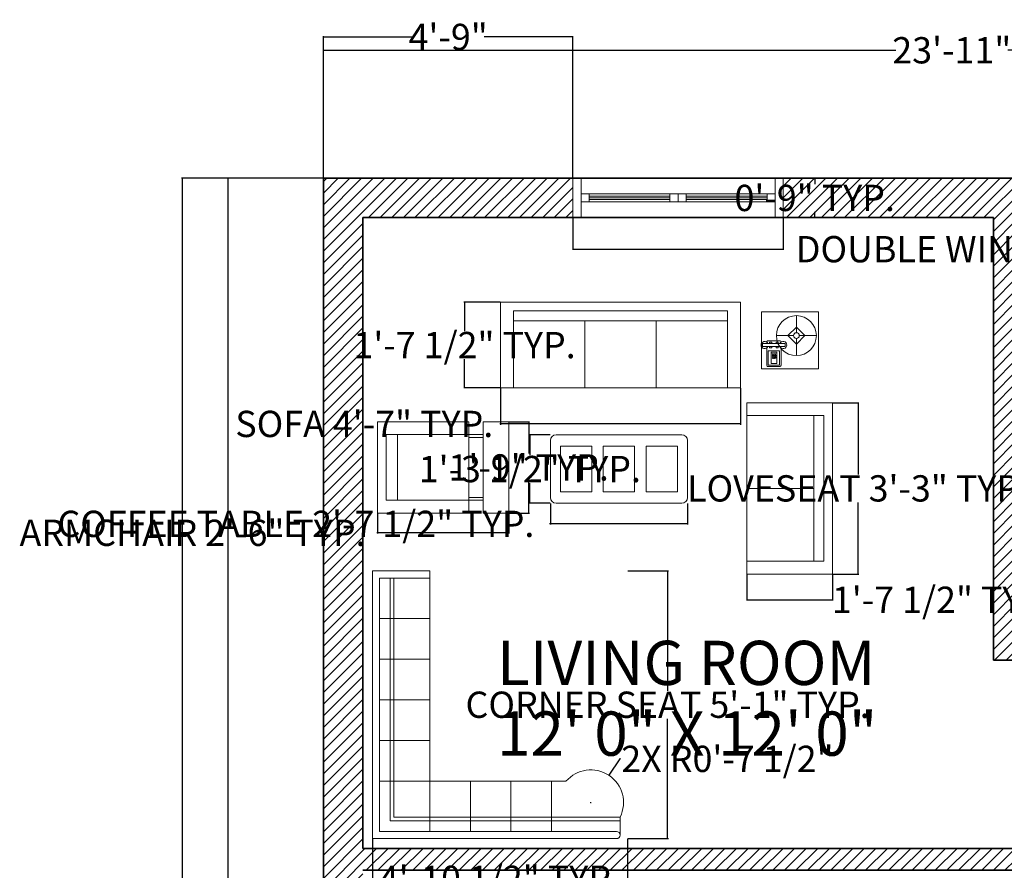
# Model space of a CAD drawing. Units: inches. Extents: x 585 to 1401, y -184 to 463.
# Tile 5 of 8: x 585 to 810, y 264 to 458. Entities that reach past the tile are written whole.
import ezdxf

# ---------------------------------------------------------------- set-up
doc = ezdxf.new("R2010")
doc.units = ezdxf.units.IN
doc.header["$MEASUREMENT"] = 0
for name, color, linetype, lineweight in [('A-ANNO-DIMS', 2, 'Continuous', 18), ('A-AREA-IDEN', 7, 'Continuous', 18), ('A-EQPM', 8, 'Continuous', 13), ('A-FURN', 8, 'Continuous', 18), ('A-Glaz', 140, 'Continuous', 18), ('A-Wall', 7, 'Continuous', 35), ('A-WALL-PATT', 252, 'Continuous', 13)]:
    doc.layers.add(name, color=color, linetype=linetype, lineweight=lineweight)
doc.styles.get("Standard").update_dxf_attribs({"font": 'arial.ttf'})
doc.dimstyles.get("Standard").update_dxf_attribs({"dimtxt": 6, "dimasz": 0.18, "dimexe": 0.18, "dimexo": 0.0625, "dimgap": 0.09, "dimtad": 0, "dimtih": 1, "dimtoh": 1, "dimdec": 0, "dimzin": 0, "dimdsep": 46, "dimlunit": 3, "dimtxsty": 'Standard', "dimblk": 'ARCHTICK', "dimcen": 0.09, "dimadec": 0, "dimazin": 0, "dimtfac": 1, "dimtdec": 0, "dimtofl": 0, "dimtmove": 0, "dimatfit": 3, "dimfxl": 1, "dimtolj": 1, "dimtzin": 0, "dimarcsym": 0})

# ---------------------------------------------------------------- blocks, each defined once
blk = doc.blocks.new('RECLIN32')
for p, q in [((16, 0), (16, -32)), ((-11.5, -3), (11.5, -3)), ((-11.5, -32), (-11.5, -3)), ((11.5, -3), (11.5, -32)), ((-11.5, -7), (11.5, -7)), ((-11.5, -32), (-11.5, -37)), ((-10.5, -32), (-10.5, -37)), ((10.5, -32), (10.5, -37)), ((11.5, -32), (11.5, -37))]:
    blk.add_line(p, q)
blk.add_lwpolyline([(16, -32), (-16, -32), (-16, 0), (16, 0)])
blk.add_lwpolyline([(-16, -46), (-16, -37), (16, -37), (16, -46)], close=True)
blk = doc.blocks.new('LOVESET5')
for p, q in [((35.75, 0), (35.75, -30.00001)), ((-19.75, -3), (31.25, -3)), ((-19.75, -30.00001), (-19.75, -3)), ((31.25, -3), (31.25, -30.00001)), ((-19.75, -6.5), (31.25, -6.5)), ((5.75, -6.5), (5.75, -30.00001))]:
    blk.add_line(p, q)
for points in [[(35.75, -30.00001), (-24.25, -30.00001), (-24.25, 0), (24.25, 0)], [(24.25, 0), (35.75, 0)]]:
    blk.add_lwpolyline(points)
blk = doc.blocks.new('TBLEN20S')
blk.add_lwpolyline([(-10, -10), (-10, 10), (10, 10), (10, -10)], close=True)
blk = doc.blocks.new('LAMP')
for p, q in [((0, 7), (0, 1)), ((-1, 0), (-7, 0)), ((0, 3), (-3, 0)), ((-3, 0), (0, -3)), ((3, 0), (0, 3)), ((0, -3), (3, 0)), ((1, 0), (7, 0)), ((0, -1), (0, -7))]:
    blk.add_line(p, q)
for radius in [7, 1]:
    blk.add_circle((0, 0), radius)
blk = doc.blocks.new('SOFA7')
for p, q in [((-37.5, -3), (37.5, -3)), ((-37.5, -30), (-37.5, -3)), ((37.5, -3), (37.5, -30)), ((-37.5, -6.5), (37.5, -6.5)), ((-12.5, -6.5), (-12.5, -30)), ((12.5, -6.5), (12.5, -30))]:
    blk.add_line(p, q)
blk.add_lwpolyline([(-42, -30), (-42, 0), (42, 0), (42, -30)], close=True)
blk = doc.blocks.new('TBLWGLAS')
for p, q in [((-22, 0), (22, 0)), ((-24, -22), (-24, -2)), ((24, -2), (24, -22)), ((-20.5, -20), (-20.5, -4)), ((-20.5, -4), (-9.5, -4)), ((-9.5, -4), (-9.5, -20)), ((-5.5, -20), (-5.5, -4)), ((-5.5, -4), (5.5, -4)), ((5.5, -4), (5.5, -20)), ((9.5, -20), (9.5, -4)), ((9.5, -4), (20.5, -4)), ((20.5, -4), (20.5, -20)), ((-9.5, -20), (-20.5, -20)), ((5.5, -20), (-5.5, -20)), ((20.5, -20), (9.5, -20)), ((22, -24), (-22, -24))]:
    blk.add_line(p, q)
for centre, start, end in [((-22, -2), 90, 180), ((22, -2), 0, 90), ((-22, -22), 180, 270), ((22, -22), 270, 0)]:
    blk.add_arc(centre, 2, start, end)
blk = doc.blocks.new('PHONE')
for p, q in [((-3.99, 3.5), (-3.99, 2.5)), ((4.01, 3.5), (-3.99, 3.5)), ((-2.02, 4.5), (2.02, 4.5)), ((-1.49, 4), (-0.74, 4)), ((-1.49, 3.5), (-1.49, 4)), ((-0.74, 4), (-0.74, 3.5)), ((0.76, 4), (0.76, 3.5)), ((1.51, 4), (0.76, 4)), ((1.51, 3.5), (1.51, 4)), ((4.01, 2.5), (4.01, 3.5)), ((-3.99, 2.5), (4.01, 2.5)), ((-2.49, -4.03), (-2.49, 1.92)), ((-1.99, 1), (-1.99, -4)), ((2.01, 1), (-1.99, 1)), ((-1.49, 2), (-1.49, 2.5)), ((-0.74, 2), (-1.49, 2)), ((1.01, 0.5), (-0.99, 0.5)), ((-0.99, 0.5), (-0.99, -3.5)), ((-0.74, 2.5), (-0.74, 2)), ((0.76, 2.5), (0.76, 2)), ((0.76, 2), (1.51, 2)), ((1.01, -3.5), (1.01, 0.5)), ((1.51, 2), (1.51, 2.5)), ((2.01, -4), (2.01, 1)), ((2.51, 1.95), (2.51, -4.06)), ((2.04, -4.5), (-2.01, -4.5)), ((-1.99, -4), (2.01, -4)), ((-0.99, -3.5), (1.01, -3.5))]:
    blk.add_line(p, q)
for centre, radius, start, end in [((-3.24, 3), 1.27, 24.0275, 336.6167), ((-2.05, 4.06), 0.442, 81.8699, 188.1301), ((2.07, 4.06), 0.442, 351.8699, 98.1301), ((3.26, 3), 1.25, 205.0096, 154.8206), ((-2.05, -4.06), 0.442, 171.8699, 278.1301), ((2.07, -4.06), 0.442, 261.8699, 8.1301)]:
    blk.add_arc(centre, radius, start, end)
blk = doc.blocks.new('QU')
at = {"color": 0}
for p, q in [((-0.8, -2.5), (-0.8, 1.233)), ((-0.8, 1.233), (0, 1.233)), ((-0.7, -2.4), (-0.7, 1.133)), ((-0.7, 1.133), (0, 1.133)), ((-0.55, -2.25), (-0.55, 1.133)), ((-0.5, -2.2), (-0.5, 1.133)), ((0, 1.233), (0, -2.4)), ((-0.7, 0.567), (0, 0.567)), ((-0.7, 0), (0, 0)), ((-0.7, -0.567), (0, -0.567)), ((-0.7, -1.133), (0, -1.133)), ((-0.7, -1.7), (1.133, -1.7)), ((-0.133, -1.7), (1.7, -1.7)), ((0.567, -1.7), (0.567, -2.4)), ((1.133, -1.7), (1.133, -2.4)), ((1.133, -1.7), (1.133, -2.4)), ((1.7, -1.7), (1.9, -1.7)), ((1.7, -1.7), (1.7, -2.4)), ((2.655, -2.25), (-0.55, -2.25)), ((2.655, -2.2), (-0.5, -2.2)), ((2.655, -2.45), (2.655, -2.2)), ((2.605, -2.4), (-0.7, -2.4)), ((2.605, -2.5), (-0.8, -2.5))]:
    blk.add_line(p, q, dxfattribs=at)
for centre, radius, start, end in [((2.247, -1.997), 0.456, 333.5922, 139.3979), ((2.605, -2.45), 0.05, 270, 90)]:
    blk.add_arc(centre, radius, start, end, dxfattribs=at)
blk = doc.blocks.new('_ArchTick')
at = {"color": 0, "linetype": 'ByBlock', "const_width": 0.15}
blk.add_lwpolyline([(-0.5, -0.5), (0.5, 0.5)], dxfattribs=at)
blk = doc.blocks.new('*D27')
at = {"layer": 'A-ANNO-DIMS', "color": 0, "lineweight": -2, "transparency": 16777216}
for p, q in [((654.47, 422.15), (632.54, 422.15)), ((632.72, 422.15), (632.72, 159.24)), ((632.72, -109.85), (632.72, 153.06)), ((654.47, -109.85), (632.54, -109.85))]:
    blk.add_line(p, q, dxfattribs=at)
at = {"layer": 'Defpoints', "color": 0, "transparency": 16777216}
for p in [(654.53, 422.15), (632.72, -109.85), (654.53, -109.85)]:
    blk.add_point(p, dxfattribs=at)
at = {"layer": 'A-ANNO-DIMS', "color": 0, "lineweight": -2, "transparency": 16777216, "xscale": 0.18, "yscale": 0.18, "zscale": 0.18}
for p, rotation in [((632.72, 422.15), 90), ((632.72, -109.85), 270)]:
    blk.add_blockref('_ArchTick', p, dxfattribs=dict(at, rotation=rotation))
at = {"layer": 'A-ANNO-DIMS', "color": 0, "transparency": 16777216, "insert": (632.72, 156.15), "char_height": 6, "attachment_point": 5}
blk.add_mtext('\\A1;44\'-4"', dxfattribs=at)
blk = doc.blocks.new('*D28')
at = {"layer": 'A-ANNO-DIMS', "color": 0, "lineweight": -2, "transparency": 16777216}
for p, q in [((654.53, 422.22), (654.53, 451.54)), ((654.53, 451.36), (785.25, 451.36)), ((941.53, 451.36), (810.81, 451.36)), ((941.53, 422.22), (941.53, 451.54))]:
    blk.add_line(p, q, dxfattribs=at)
at = {"layer": 'Defpoints', "color": 0, "transparency": 16777216}
for p in [(941.53, 451.36), (654.53, 422.15), (941.53, 422.15)]:
    blk.add_point(p, dxfattribs=at)
at = {"layer": 'A-ANNO-DIMS', "color": 0, "lineweight": -2, "transparency": 16777216, "xscale": 0.18, "yscale": 0.18, "zscale": 0.18, "rotation": 180}
blk.add_blockref('_ArchTick', (654.53, 451.36), dxfattribs=at)
at = {"layer": 'A-ANNO-DIMS', "color": 0, "lineweight": -2, "transparency": 16777216, "xscale": 0.18, "yscale": 0.18, "zscale": 0.18}
blk.add_blockref('_ArchTick', (941.53, 451.36), dxfattribs=at)
at = {"layer": 'A-ANNO-DIMS', "color": 0, "transparency": 16777216, "insert": (798.03, 451.36), "char_height": 6, "attachment_point": 5}
blk.add_mtext('\\A1;23\'-11"', dxfattribs=at)
blk = doc.blocks.new('WIN-48-DOUBLE-PANEL')
for p, q in [((48, 9), (0, 9)), ((0, 9), (0, 0)), ((1.85, 9), (0, 9)), ((0, 9), (0, 0)), ((1.85, 0), (1.85, 9)), ((1.85, 0), (1.85, 9)), ((46.15, 9), (48, 9)), ((46.15, 0), (46.15, 9)), ((46.15, 0), (46.15, 9)), ((46.15, 0), (46.15, 9)), ((48, 9), (48, 0)), ((48, 0), (48, 9)), ((1.85, 5.44), (46.15, 5.44)), ((3.69, 3.6), (3.69, 5.44)), ((3.69, 4.89), (22.15, 4.89)), ((3.69, 4.52), (22.15, 4.52)), ((22.15, 5.44), (22.15, 3.6)), ((24, 5.44), (24, 3.6)), ((25.85, 5.44), (25.85, 3.6)), ((44.31, 4.89), (25.85, 4.89)), ((44.31, 4.52), (25.85, 4.52)), ((44.31, 3.6), (44.31, 5.44)), ((1.85, 3.6), (46.15, 3.6)), ((3.69, 4.15), (22.15, 4.15)), ((44.31, 4.15), (25.85, 4.15)), ((0, 0), (1.85, 0)), ((48, 0), (0, 0)), ((48, 0), (46.15, 0))]:
    blk.add_line(p, q)
blk = doc.blocks.new('TELEPHONE-KEYPAD')
for centre in [(0.08, 1.02), (0.11, 0.71), (0.14, 0.39), (0.15, 0.09), (0.39, 1.03), (0.42, 0.71), (0.41, 0.38), (0.44, 0.08), (0.73, 1.02), (0.74, 0.7), (0.75, 0.4), (0.76, 0.13)]:
    blk.add_circle(centre, 0.0754)
blk = doc.blocks.new('*D38')
at = {"layer": 'A-ANNO-DIMS', "color": 0, "lineweight": -2, "transparency": 16777216}
for p, q in [((711.53, 413.09), (711.53, 405.77)), ((759.53, 413.09), (759.53, 405.77)), ((711.53, 405.95), (759.53, 405.95)), ((759.53, 405.95), (759.71, 405.95))]:
    blk.add_line(p, q, dxfattribs=at)
at = {"layer": 'Defpoints', "color": 0, "transparency": 16777216}
for p in [(711.53, 413.15), (759.53, 413.15), (759.53, 405.95)]:
    blk.add_point(p, dxfattribs=at)
at = {"layer": 'A-ANNO-DIMS', "color": 0, "lineweight": -2, "transparency": 16777216, "xscale": 0.18, "yscale": 0.18, "zscale": 0.18, "rotation": 180}
blk.add_blockref('_ArchTick', (711.53, 405.95), dxfattribs=at)
at = {"layer": 'A-ANNO-DIMS', "color": 0, "lineweight": -2, "transparency": 16777216, "xscale": 0.18, "yscale": 0.18, "zscale": 0.18}
blk.add_blockref('_ArchTick', (759.53, 405.95), dxfattribs=at)
at = {"layer": 'A-ANNO-DIMS', "color": 0, "transparency": 16777216, "insert": (815.89, 405.95), "char_height": 6, "attachment_point": 5}
blk.add_mtext('\\A1;DOUBLE WINDOW 4\'-0" TYP.', dxfattribs=at)
blk = doc.blocks.new('*D39')
at = {"layer": 'A-ANNO-DIMS', "color": 0, "lineweight": -2, "transparency": 16777216}
for p, q in [((759.59, 422.15), (766.91, 422.15)), ((766.73, 422.15), (766.73, 420.81)), ((766.73, 413.15), (766.73, 414.5)), ((759.59, 413.15), (766.91, 413.15))]:
    blk.add_line(p, q, dxfattribs=at)
at = {"layer": 'Defpoints', "color": 0, "transparency": 16777216}
for p in [(759.53, 422.15), (766.73, 422.15), (759.53, 413.15)]:
    blk.add_point(p, dxfattribs=at)
at = {"layer": 'A-ANNO-DIMS', "color": 0, "lineweight": -2, "transparency": 16777216, "xscale": 0.18, "yscale": 0.18, "zscale": 0.18}
for p, rotation in [((766.73, 422.15), 90), ((766.73, 413.15), 270)]:
    blk.add_blockref('_ArchTick', p, dxfattribs=dict(at, rotation=rotation))
at = {"layer": 'A-ANNO-DIMS', "color": 0, "transparency": 16777216, "insert": (766.73, 417.65), "char_height": 6, "attachment_point": 5}
blk.add_mtext('\\A1;0\'-9" TYP.', dxfattribs=at)
blk = doc.blocks.new('*D48')
at = {"layer": 'A-ANNO-DIMS', "color": 0, "lineweight": -2, "transparency": 16777216}
for p, q in [((666.91, 345.64), (666.91, 341.02)), ((696.91, 345.64), (696.91, 341.02)), ((666.91, 341.2), (666.73, 341.2)), ((696.91, 341.2), (666.91, 341.2))]:
    blk.add_line(p, q, dxfattribs=at)
at = {"layer": 'Defpoints', "color": 0, "transparency": 16777216}
for p in [(666.91, 345.7), (696.91, 345.7), (666.91, 341.2)]:
    blk.add_point(p, dxfattribs=at)
at = {"layer": 'A-ANNO-DIMS', "color": 0, "lineweight": -2, "transparency": 16777216, "xscale": 0.18, "yscale": 0.18, "zscale": 0.18, "rotation": 180.0000000000005}
blk.add_blockref('_ArchTick', (666.91, 341.2), dxfattribs=at)
at = {"layer": 'A-ANNO-DIMS', "color": 0, "lineweight": -2, "transparency": 16777216, "xscale": 0.18, "yscale": 0.18, "zscale": 0.18}
blk.add_blockref('_ArchTick', (696.91, 341.2), dxfattribs=at)
at = {"layer": 'A-ANNO-DIMS', "color": 0, "transparency": 16777216, "insert": (624.66, 341.2), "char_height": 6, "attachment_point": 5}
blk.add_mtext('\\A1;ARMCHAIR 2\'-6" TYP.', dxfattribs=at)
blk = doc.blocks.new('*D49')
at = {"layer": 'A-ANNO-DIMS', "color": 0, "lineweight": -2, "transparency": 16777216}
for p, q in [((696.97, 366.57), (701.59, 366.57)), ((701.41, 366.57), (701.41, 359.29)), ((701.41, 345.7), (701.41, 352.98)), ((696.97, 345.7), (701.59, 345.7))]:
    blk.add_line(p, q, dxfattribs=at)
at = {"layer": 'Defpoints', "color": 0, "transparency": 16777216}
for p in [(696.91, 366.57), (696.91, 345.7), (701.41, 345.7)]:
    blk.add_point(p, dxfattribs=at)
at = {"layer": 'A-ANNO-DIMS', "color": 0, "lineweight": -2, "transparency": 16777216, "xscale": 0.18, "yscale": 0.18, "zscale": 0.18}
for p, rotation in [((701.41, 366.57), 90), ((701.41, 345.7), 270)]:
    blk.add_blockref('_ArchTick', p, dxfattribs=dict(at, rotation=rotation))
at = {"layer": 'A-ANNO-DIMS', "color": 0, "transparency": 16777216, "insert": (701.41, 356.13), "char_height": 6, "attachment_point": 5}
blk.add_mtext('\\A1;1\'-9" TYP.', dxfattribs=at)
blk = doc.blocks.new('*D50')
at = {"layer": 'A-ANNO-DIMS', "color": 0, "lineweight": -2, "transparency": 16777216}
for p, q in [((770.82, 370.91), (776.81, 370.91)), ((776.63, 370.91), (776.63, 354.54)), ((776.63, 331.78), (776.63, 348.14)), ((770.82, 331.78), (776.81, 331.78))]:
    blk.add_line(p, q, dxfattribs=at)
at = {"layer": 'Defpoints', "color": 0, "transparency": 16777216}
for p in [(770.76, 370.91), (776.63, 370.91), (770.76, 331.78)]:
    blk.add_point(p, dxfattribs=at)
at = {"layer": 'A-ANNO-DIMS', "color": 0, "lineweight": -2, "transparency": 16777216, "xscale": 0.18, "yscale": 0.18, "zscale": 0.18}
for p, rotation in [((776.63, 370.91), 90), ((776.63, 331.78), 270)]:
    blk.add_blockref('_ArchTick', p, dxfattribs=dict(at, rotation=rotation))
at = {"layer": 'A-ANNO-DIMS', "color": 0, "transparency": 16777216, "insert": (776.63, 351.34), "char_height": 6, "attachment_point": 5}
blk.add_mtext('\\A1;LOVESEAT 3\'-3" TYP.', dxfattribs=at)
blk = doc.blocks.new('*D51')
at = {"layer": 'A-ANNO-DIMS', "color": 0, "lineweight": -2, "transparency": 16777216}
for p, q in [((751.2, 331.71), (751.2, 325.73)), ((770.76, 331.71), (770.76, 325.73)), ((751.2, 325.91), (770.76, 325.91)), ((770.76, 325.91), (770.94, 325.91))]:
    blk.add_line(p, q, dxfattribs=at)
at = {"layer": 'Defpoints', "color": 0, "transparency": 16777216}
for p in [(751.2, 331.78), (770.76, 331.78), (770.76, 325.91)]:
    blk.add_point(p, dxfattribs=at)
at = {"layer": 'A-ANNO-DIMS', "color": 0, "lineweight": -2, "transparency": 16777216, "xscale": 0.18, "yscale": 0.18, "zscale": 0.18, "rotation": 180}
blk.add_blockref('_ArchTick', (751.2, 325.91), dxfattribs=at)
at = {"layer": 'A-ANNO-DIMS', "color": 0, "lineweight": -2, "transparency": 16777216, "xscale": 0.18, "yscale": 0.18, "zscale": 0.18}
blk.add_blockref('_ArchTick', (770.76, 325.91), dxfattribs=at)
at = {"layer": 'A-ANNO-DIMS', "color": 0, "transparency": 16777216, "insert": (796.03, 325.91), "char_height": 6, "attachment_point": 5}
blk.add_mtext('\\A1;1\'-7 1/2" TYP.', dxfattribs=at)
blk = doc.blocks.new('*D56')
at = {"layer": 'A-ANNO-DIMS', "color": 0, "lineweight": -2, "transparency": 16777216}
for p, q in [((694.99, 374.21), (694.99, 365.88)), ((749.77, 374.21), (749.77, 365.88)), ((694.99, 366.06), (694.81, 366.06)), ((749.77, 366.06), (694.99, 366.06))]:
    blk.add_line(p, q, dxfattribs=at)
at = {"layer": 'Defpoints', "color": 0, "transparency": 16777216}
for p in [(694.99, 374.27), (749.77, 374.27), (694.99, 366.06)]:
    blk.add_point(p, dxfattribs=at)
at = {"layer": 'A-ANNO-DIMS', "color": 0, "lineweight": -2, "transparency": 16777216, "xscale": 0.18, "yscale": 0.18, "zscale": 0.18, "rotation": 180}
blk.add_blockref('_ArchTick', (694.99, 366.06), dxfattribs=at)
at = {"layer": 'A-ANNO-DIMS', "color": 0, "lineweight": -2, "transparency": 16777216, "xscale": 0.18, "yscale": 0.18, "zscale": 0.18}
blk.add_blockref('_ArchTick', (749.77, 366.06), dxfattribs=at)
at = {"layer": 'A-ANNO-DIMS', "color": 0, "transparency": 16777216, "insert": (663.87, 366.06), "char_height": 6, "attachment_point": 5}
blk.add_mtext('\\A1;SOFA 4\'-7" TYP.', dxfattribs=at)
blk = doc.blocks.new('*D57')
at = {"layer": 'A-ANNO-DIMS', "color": 0, "lineweight": -2, "transparency": 16777216}
for p, q in [((694.93, 393.84), (686.59, 393.84)), ((686.77, 393.84), (686.77, 387.25)), ((686.77, 374.27), (686.77, 380.86)), ((694.93, 374.27), (686.59, 374.27))]:
    blk.add_line(p, q, dxfattribs=at)
at = {"layer": 'Defpoints', "color": 0, "transparency": 16777216}
for p in [(686.77, 393.84), (694.99, 393.84), (694.99, 374.27)]:
    blk.add_point(p, dxfattribs=at)
at = {"layer": 'A-ANNO-DIMS', "color": 0, "lineweight": -2, "transparency": 16777216, "xscale": 0.18, "yscale": 0.18, "zscale": 0.18}
for p, rotation in [((686.77, 393.84), 90), ((686.77, 374.27), 270)]:
    blk.add_blockref('_ArchTick', p, dxfattribs=dict(at, rotation=rotation))
at = {"layer": 'A-ANNO-DIMS', "color": 0, "transparency": 16777216, "insert": (686.77, 384.06), "char_height": 6, "attachment_point": 5}
blk.add_mtext('\\A1;1\'-7 1/2" TYP.', dxfattribs=at)
blk = doc.blocks.new('*D58')
at = {"layer": 'A-ANNO-DIMS', "color": 0, "lineweight": -2, "transparency": 16777216}
for p, q in [((706.37, 347.87), (706.37, 343.06)), ((737.67, 347.87), (737.67, 343.06)), ((706.37, 343.24), (706.19, 343.24)), ((737.67, 343.24), (706.37, 343.24))]:
    blk.add_line(p, q, dxfattribs=at)
at = {"layer": 'Defpoints', "color": 0, "transparency": 16777216}
for p in [(706.37, 347.93), (737.67, 347.93), (706.37, 343.24)]:
    blk.add_point(p, dxfattribs=at)
at = {"layer": 'A-ANNO-DIMS', "color": 0, "lineweight": -2, "transparency": 16777216, "xscale": 0.18, "yscale": 0.18, "zscale": 0.18, "rotation": 180}
blk.add_blockref('_ArchTick', (706.37, 343.24), dxfattribs=at)
at = {"layer": 'A-ANNO-DIMS', "color": 0, "lineweight": -2, "transparency": 16777216, "xscale": 0.18, "yscale": 0.18, "zscale": 0.18}
blk.add_blockref('_ArchTick', (737.67, 343.24), dxfattribs=at)
at = {"layer": 'A-ANNO-DIMS', "color": 0, "transparency": 16777216, "insert": (648.25, 343.24), "char_height": 6, "attachment_point": 5}
blk.add_mtext('\\A1;COFFEE TABLE 2\'-7 1/2" TYP.', dxfattribs=at)
blk = doc.blocks.new('*D59')
at = {"layer": 'A-ANNO-DIMS', "color": 0, "lineweight": -2, "transparency": 16777216}
for p, q in [((706.3, 363.59), (701.49, 363.59)), ((701.67, 363.59), (701.67, 358.95)), ((701.67, 347.93), (701.67, 352.57)), ((706.3, 347.93), (701.49, 347.93))]:
    blk.add_line(p, q, dxfattribs=at)
at = {"layer": 'Defpoints', "color": 0, "transparency": 16777216}
for p in [(701.67, 363.59), (706.37, 363.59), (706.37, 347.93)]:
    blk.add_point(p, dxfattribs=at)
at = {"layer": 'A-ANNO-DIMS', "color": 0, "lineweight": -2, "transparency": 16777216, "xscale": 0.18, "yscale": 0.18, "zscale": 0.18}
for p, rotation in [((701.67, 363.59), 90), ((701.67, 347.93), 270)]:
    blk.add_blockref('_ArchTick', p, dxfattribs=dict(at, rotation=rotation))
at = {"layer": 'A-ANNO-DIMS', "color": 0, "transparency": 16777216, "insert": (701.67, 355.76), "char_height": 6, "attachment_point": 5}
blk.add_mtext('\\A1;1\'-3 1/2" TYP.', dxfattribs=at)
blk = doc.blocks.new('*D64')
at = {"layer": 'A-ANNO-DIMS', "color": 0, "lineweight": -2, "transparency": 16777216}
for p, q in [((724.03, 332.51), (733.32, 332.51)), ((733.14, 332.51), (733.14, 305.14)), ((733.14, 271.38), (733.14, 298.75)), ((724.03, 271.38), (733.32, 271.38))]:
    blk.add_line(p, q, dxfattribs=at)
at = {"layer": 'Defpoints', "color": 0, "transparency": 16777216}
for p in [(723.97, 332.51), (733.14, 332.51), (723.97, 271.38)]:
    blk.add_point(p, dxfattribs=at)
at = {"layer": 'A-ANNO-DIMS', "color": 0, "lineweight": -2, "transparency": 16777216, "xscale": 0.18, "yscale": 0.18, "zscale": 0.18}
for p, rotation in [((733.14, 332.51), 90), ((733.14, 271.38), 270)]:
    blk.add_blockref('_ArchTick', p, dxfattribs=dict(at, rotation=rotation))
at = {"layer": 'A-ANNO-DIMS', "color": 0, "transparency": 16777216, "insert": (733.14, 301.95), "char_height": 6, "attachment_point": 5}
blk.add_mtext('\\A1;CORNER SEAT 5\'-1" TYP.', dxfattribs=at)
blk = doc.blocks.new('*D65')
at = {"layer": 'A-ANNO-DIMS', "color": 0, "lineweight": -2, "transparency": 16777216}
for p, q in [((665.71, 271.32), (665.71, 262.03)), ((723.97, 271.32), (723.97, 262.03)), ((665.71, 262.21), (667.02, 262.21)), ((723.97, 262.21), (722.66, 262.21))]:
    blk.add_line(p, q, dxfattribs=at)
at = {"layer": 'Defpoints', "color": 0, "transparency": 16777216}
for p in [(665.71, 271.38), (723.97, 271.38), (723.97, 262.21)]:
    blk.add_point(p, dxfattribs=at)
at = {"layer": 'A-ANNO-DIMS', "color": 0, "lineweight": -2, "transparency": 16777216, "xscale": 0.18, "yscale": 0.18, "zscale": 0.18, "rotation": 180}
blk.add_blockref('_ArchTick', (665.71, 262.21), dxfattribs=at)
at = {"layer": 'A-ANNO-DIMS', "color": 0, "lineweight": -2, "transparency": 16777216, "xscale": 0.18, "yscale": 0.18, "zscale": 0.18}
blk.add_blockref('_ArchTick', (723.97, 262.21), dxfattribs=at)
at = {"layer": 'A-ANNO-DIMS', "color": 0, "transparency": 16777216, "insert": (694.84, 262.21), "char_height": 6, "attachment_point": 5}
blk.add_mtext('\\A1;4\'-10 1/2" TYP.', dxfattribs=at)
blk = doc.blocks.new('*D76')
at = {"layer": 'A-ANNO-DIMS', "color": 0, "lineweight": -2, "transparency": 16777216}
for p, q in [((654.47, 422.15), (622.1, 422.15)), ((622.28, 422.15), (622.28, 142.65)), ((622.28, -143.23), (622.28, 136.27)), ((807.47, -143.23), (622.1, -143.23))]:
    blk.add_line(p, q, dxfattribs=at)
at = {"layer": 'Defpoints', "color": 0, "transparency": 16777216}
for p in [(622.28, 422.15), (654.53, 422.15), (807.53, -143.23)]:
    blk.add_point(p, dxfattribs=at)
at = {"layer": 'A-ANNO-DIMS', "color": 0, "lineweight": -2, "transparency": 16777216, "xscale": 0.18, "yscale": 0.18, "zscale": 0.18}
for p, rotation in [((622.28, 422.15), 90), ((622.28, -143.23), 270)]:
    blk.add_blockref('_ArchTick', p, dxfattribs=dict(at, rotation=rotation))
at = {"layer": 'A-ANNO-DIMS', "color": 0, "transparency": 16777216, "insert": (622.28, 139.46), "char_height": 6, "attachment_point": 5}
blk.add_mtext('\\A1;47\'-1 1/2"', dxfattribs=at)
blk = doc.blocks.new('*D82')
at = {"layer": 'A-ANNO-DIMS', "color": 0, "lineweight": -2, "transparency": 16777216}
for p, q in [((654.53, 422.22), (654.53, 454.58)), ((654.53, 454.4), (674.84, 454.4)), ((711.53, 454.4), (691.21, 454.4)), ((711.53, 422.22), (711.53, 454.58))]:
    blk.add_line(p, q, dxfattribs=at)
at = {"layer": 'Defpoints', "color": 0, "transparency": 16777216}
for p in [(711.53, 454.4), (654.53, 422.15), (711.53, 422.15)]:
    blk.add_point(p, dxfattribs=at)
at = {"layer": 'A-ANNO-DIMS', "color": 0, "lineweight": -2, "transparency": 16777216, "xscale": 0.18, "yscale": 0.18, "zscale": 0.18, "rotation": 180}
blk.add_blockref('_ArchTick', (654.53, 454.4), dxfattribs=at)
at = {"layer": 'A-ANNO-DIMS', "color": 0, "lineweight": -2, "transparency": 16777216, "xscale": 0.18, "yscale": 0.18, "zscale": 0.18}
blk.add_blockref('_ArchTick', (711.53, 454.4), dxfattribs=at)
at = {"layer": 'A-ANNO-DIMS', "color": 0, "transparency": 16777216, "insert": (683.03, 454.4), "char_height": 6, "attachment_point": 5}
blk.add_mtext('\\A1;4\'-9"', dxfattribs=at)
blk = doc.blocks.new('*D98')
at = {"layer": 'A-ANNO-DIMS', "color": 0, "lineweight": -2, "transparency": 16777216}
for p, q in [((722.2, 289.59), (719.72, 285.85)), ((722.38, 289.59), (722.2, 289.59)), ((715.51, 279.62), (715.69, 279.62)), ((715.6, 279.53), (715.6, 279.71))]:
    blk.add_line(p, q, dxfattribs=at)
at = {"layer": 'Defpoints', "color": 0, "transparency": 16777216}
for p in [(719.72, 285.85), (715.6, 279.62)]:
    blk.add_point(p, dxfattribs=at)
at = {"layer": 'A-ANNO-DIMS', "color": 0, "lineweight": -2, "transparency": 16777216, "xscale": 0.18, "yscale": 0.18, "zscale": 0.18, "rotation": 236.4909758134295}
blk.add_blockref('_ArchTick', (719.72, 285.85), dxfattribs=at)
at = {"layer": 'A-ANNO-DIMS', "color": 0, "transparency": 16777216, "insert": (746.8, 289.59), "char_height": 6, "attachment_point": 5}
blk.add_mtext('\\A1;2X R0\'-7 1/2"', dxfattribs=at)

msp = doc.modelspace()

# ---------------------------------------------------------------- hatches: boundary and pattern name
at = {"layer": 'A-WALL-PATT'}
h = msp.add_hatch(dxfattribs=at)
h.set_pattern_fill('ANSI31', color=256, scale=15)
h.set_pattern_definition([(45, (599.059, -1e-14), (-1.325825, 1.325825), [])])
h.paths.add_polyline_path([(711.53, 422.15), (654.53, 422.15), (654.53, -109.85), (680.03, -109.85), (680.03, -100.85), (663.53, -100.85), (663.53, 48.87), (759.53, 48.87), (759.53, 57.87), (663.53, 57.87), (663.53, 144.15), (663.53, 264.15), (812.53, 264.15), (812.53, 269.15), (663.53, 269.15), (663.53, 413.15), (711.53, 413.15)])
h.paths.add_polyline_path([(753.53, -100.85), (728.03, -100.85), (728.03, -109.85), (753.53, -109.85)], flags=17)
h.paths.add_polyline_path([(812.53, -71.54), (807.53, -71.54), (807.53, -100.85), (795.53, -100.85), (795.53, -109.85), (807.53, -109.85), (807.53, -143.23), (848.53, -143.23), (848.53, -134.23), (812.53, -134.23)])
h.paths.add_polyline_path([(941.53, 8.77), (932.53, 8.77), (932.53, -9.23), (812.53, -9.23), (812.53, 5.77), (807.53, 5.77), (807.53, -29.54), (812.53, -29.54), (812.53, -14.23), (932.53, -14.23), (932.53, -134.23), (896.53, -134.23), (896.53, -143.23), (941.53, -143.23)])
h.paths.add_polyline_path([(941.53, 91.77), (932.53, 91.77), (932.53, 55.77), (812.53, 55.77), (812.53, 98.58), (807.53, 98.58), (807.53, 35.77), (812.53, 35.77), (812.53, 50.77), (932.53, 50.77), (932.53, 32.77), (941.53, 32.77)])
h.paths.add_polyline_path([(941.53, 222.04), (932.53, 222.04), (932.53, 180.77), (807.53, 180.77), (807.53, 140.58), (812.53, 140.58), (812.53, 175.77), (932.53, 175.77), (932.53, 139.77), (941.53, 139.77)])
h.paths.add_polyline_path([(941.53, 422.15), (896.53, 422.15), (896.53, 413.15), (932.53, 413.15), (932.53, 317.15), (896.53, 317.15), (896.53, 312.15), (932.53, 312.15), (932.53, 270.04), (941.53, 270.04)])
h.paths.add_polyline_path([(848.53, 422.15), (759.53, 422.15), (759.53, 413.15), (807.53, 413.15), (807.53, 312.15), (848.53, 312.15), (848.53, 317.15), (812.53, 317.15), (812.53, 413.15), (848.53, 413.15)])

# ---------------------------------------------------------------- linework, layer by layer
at = {"layer": 'A-Wall'}
for p, q in [((654.53, 422.15), (654.53, -109.85)), ((654.53, 422.15), (941.53, 422.15)), ((663.53, 413.15), (663.53, 269.15)), ((663.53, 413.15), (807.53, 413.15)), ((807.53, 413.15), (807.53, 312.15)), ((807.53, 312.15), (848.53, 312.15)), ((663.53, 269.15), (812.53, 269.15)), ((663.53, 264.15), (812.53, 264.15))]:
    msp.add_line(p, q, dxfattribs=at)

# ---------------------------------------------------------------- block references
at = {"layer": 'A-EQPM', "extrusion": (0, 0, -1), "xscale": 0.6521559011617164, "yscale": 0.6521559011617164, "zscale": -0.6521559011617158}
for name, p in [('LAMP', (-762.55, 386.22)), ('PHONE', (-757.42, 382.11))]:
    msp.add_blockref(name, p, dxfattribs=at)
at = {"layer": 'A-EQPM'}
msp.add_blockref('TELEPHONE-KEYPAD', (757.03, 381), dxfattribs=at)
at = {"layer": 'A-FURN', "extrusion": (0, 0, -1), "xscale": 0.6521559011617164, "yscale": 0.6521559011617164, "zscale": -0.6521559011617158}
for name, p in [('SOFA7', (-722.38, 393.84)), ('TBLEN20S', (-761.1, 385.13)), ('TBLWGLAS', (-722.02, 363.59))]:
    msp.add_blockref(name, p, dxfattribs=at)
at = {"layer": 'A-FURN', "extrusion": (0, 0, -1), "xscale": 0.6521559011617244, "yscale": 0.6521559011617244, "zscale": -0.6521559011617158}
for name, p, rotation in [('LOVESET5', (-770.76, 347.59), 89.99999999999947), ('RECLIN32', (-666.91, 356.13), 269.9999999999994)]:
    msp.add_blockref(name, p, dxfattribs=dict(at, rotation=rotation))
at = {"layer": 'A-FURN', "xscale": 16.37472381684798, "yscale": 16.37472381684798, "zscale": 16.37472381684798}
msp.add_blockref('QU', (678.81, 312.32), dxfattribs=at)
at = {"layer": 'A-Glaz'}
msp.add_blockref('WIN-48-DOUBLE-PANEL', (711.53, 413.15), dxfattribs=at)

# ---------------------------------------------------------------- texts
at = {"layer": 'A-AREA-IDEN'}
for s, p in [('LIVING ROOM', (694.18, 306.45)), ('12\' 0" X 12\' 0"', (694.18, 290.31))]:
    msp.add_text(s, height=10.1013, dxfattribs=at).set_placement(p)

# ---------------------------------------------------------------- dimensions: what is measured, and where the dimension line sits
at = {"layer": 'A-ANNO-DIMS'}
for base, p2, override, picture, middle in [((711.53, 454.4), (711.53, 422.15), {"dimdec": 1, "dimlfac": 1, "dimrnd": 0, "dimzin": 1, "dimdsep": 46, "dimlunit": 4, "dimfrac": 2}, '*D82', (683.03, 454.4)), ((941.53, 451.36), (941.53, 422.15), {"dimclrd": 0, "dimclre": 0, "dimclrt": 0}, '*D28', (798.03, 451.36))]:
    dim = msp.add_linear_dim(base=base, p1=(654.53, 422.15), p2=p2, dimstyle='Standard', override=override, dxfattribs=at)
    dim.commit()
    dim.dimension.update_dxf_attribs({"geometry": picture, "text_midpoint": middle})
for base, p1, p2, angle, text, picture, middle in [((766.73, 422.15), (759.53, 413.15), (759.53, 422.15), 90, '<> TYP.', '*D39', (766.73, 417.65)), ((686.77, 393.84), (694.99, 374.27), (694.99, 393.84), 90, '<> TYP.', '*D57', (686.77, 384.06)), ((694.99, 366.06), (749.77, 374.27), (694.99, 374.27), 180, 'SOFA <> TYP.', '*D56', (663.87, 366.06)), ((776.63, 370.91), (770.76, 331.78), (770.76, 370.91), 90, 'LOVESEAT <> TYP.', '*D50', (776.63, 351.34)), ((701.67, 363.59), (706.37, 347.93), (706.37, 363.59), 90, '<> TYP.', '*D59', (701.67, 355.76)), ((706.37, 343.24), (737.67, 347.93), (706.37, 347.93), 180, 'COFFEE TABLE <> TYP.', '*D58', (648.25, 343.24)), ((701.41, 345.7), (696.91, 366.57), (696.91, 345.7), 270, '<> TYP.', '*D49', (701.41, 356.13)), ((666.91, 341.2), (696.91, 345.7), (666.91, 345.7), 180, 'ARMCHAIR <> TYP.', '*D48', (624.66, 341.2)), ((770.76, 325.91), (751.2, 331.78), (770.76, 331.78), 0, '<> TYP.', '*D51', (796.03, 325.91)), ((733.14, 332.51), (723.97, 271.38), (723.97, 332.51), 90, 'CORNER SEAT <> TYP.', '*D64', (733.14, 301.95))]:
    dim = msp.add_linear_dim(base=base, p1=p1, p2=p2, angle=angle, text=text, dimstyle='Standard', override={"dimdec": 1, "dimlfac": 1, "dimrnd": 0, "dimzin": 1, "dimdsep": 46, "dimlunit": 4, "dimfrac": 2}, dxfattribs=at)
    dim.commit()
    dim.dimension.update_dxf_attribs({"geometry": picture, "text_midpoint": middle})
for base, p1, p2, text, picture, middle in [((759.53, 405.95), (711.53, 413.15), (759.53, 413.15), 'DOUBLE WINDOW <> TYP.', '*D38', (815.89, 405.95)), ((723.97, 262.21), (665.71, 271.38), (723.97, 271.38), '<> TYP.', '*D65', (694.84, 262.21))]:
    dim = msp.add_linear_dim(base=base, p1=p1, p2=p2, text=text, dimstyle='Standard', override={"dimdec": 1, "dimlfac": 1, "dimrnd": 0, "dimzin": 1, "dimdsep": 46, "dimlunit": 4, "dimfrac": 2}, dxfattribs=at)
    dim.commit()
    dim.dimension.update_dxf_attribs({"geometry": picture, "text_midpoint": middle})
for base, p1, p2, override, picture, middle in [((622.28, 422.15), (807.53, -143.23), (654.53, 422.15), {"dimdec": 1, "dimlfac": 1, "dimrnd": 0, "dimzin": 1, "dimdsep": 46, "dimlunit": 4, "dimfrac": 2}, '*D76', (622.28, 139.46)), ((632.72, -109.85), (654.53, 422.15), (654.53, -109.85), {"dimclrd": 0, "dimclre": 0, "dimclrt": 0}, '*D27', (632.72, 156.15))]:
    dim = msp.add_linear_dim(base=base, p1=p1, p2=p2, angle=90, dimstyle='Standard', override=override, dxfattribs=at)
    dim.commit()
    dim.dimension.update_dxf_attribs({"geometry": picture, "text_midpoint": middle})
dim = msp.add_radius_dim(center=(715.6, 279.62), mpoint=(719.72, 285.85), text='2X <>', dimstyle='Standard', override={"dimdec": 1, "dimlfac": 1, "dimrnd": 0, "dimzin": 1, "dimdsep": 46, "dimlunit": 4, "dimfrac": 2}, dxfattribs=at)
dim.commit()
dim.dimension.update_dxf_attribs({"geometry": '*D98', "text_midpoint": (746.8, 289.59), "dimtype": 164})

doc.saveas('drawing.dxf')
